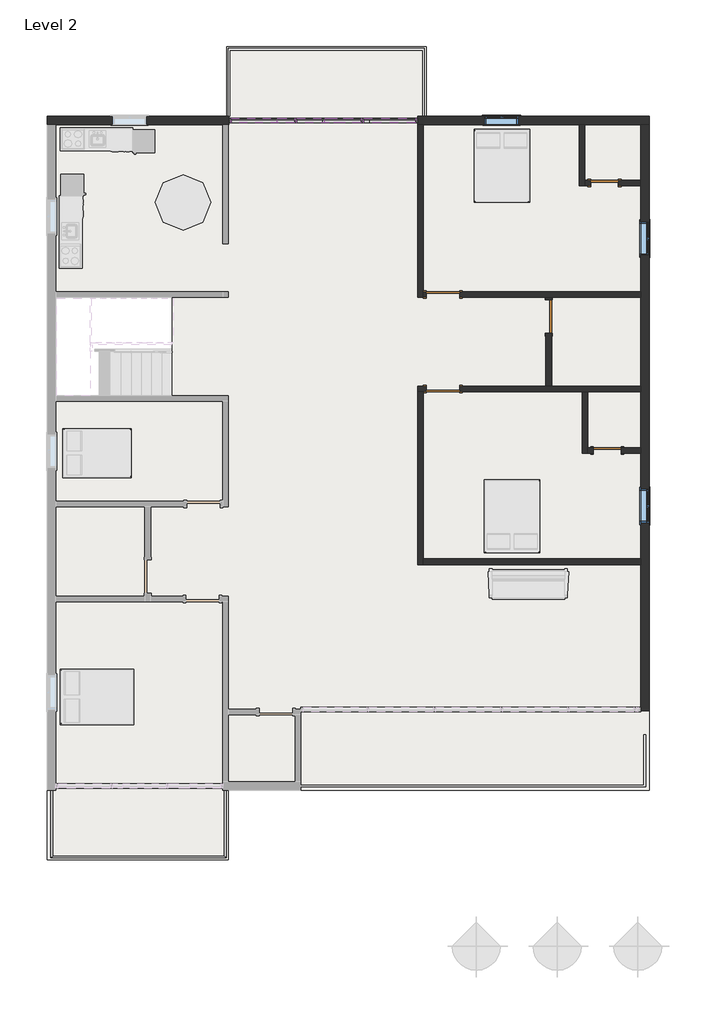
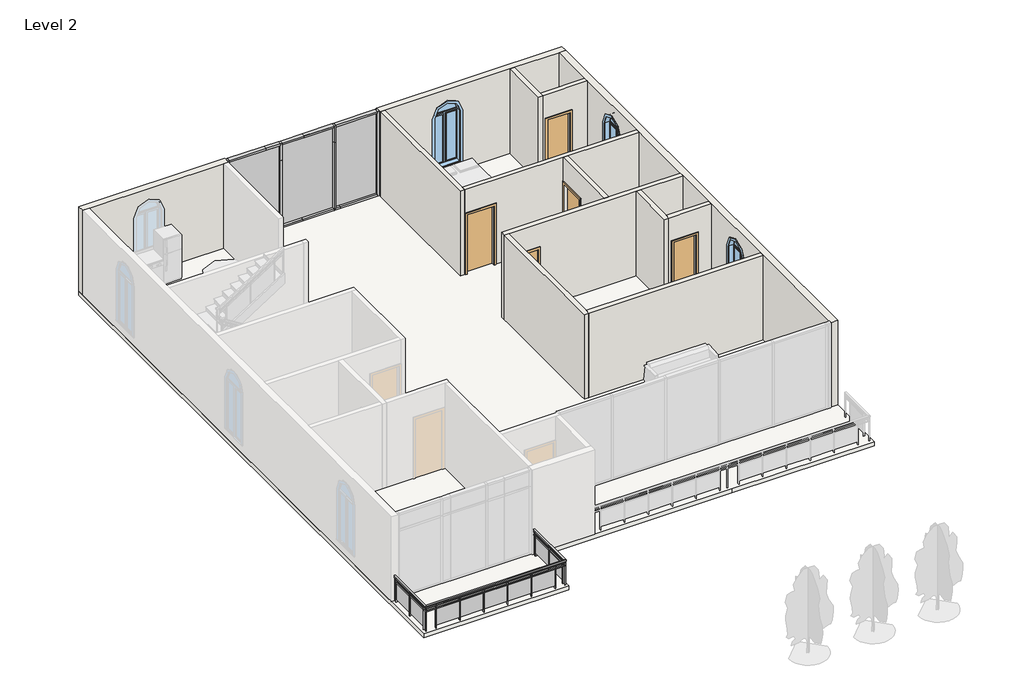
# One storey, part 2 of 3: 16 members, 13 walls, 5 doors, 3 plates, 3 windows, 1 railing, 1 slab.
"""IFC4 building model written with IfcOpenShell, lengths in millimetres."""

from ifc_helpers import new_model, si_unit, frame, origin, place, context, project, spatial, polyline, circle_curve, outline, extrude, faceted_brep, transform, mapped, element, save
from ifc_brep_helpers import plane_surface, revolved_surface, advanced_brep
from components import single_flush_2_5_e2b13fe9, door_686f89d2, door_16372e1c, member_f0fea5a5, member_f3b54ad7, member_8346ef35, member_675b1c02, member_6ed1261f, member_2238a540, member_64ee9188, member_6d5c3e5e, member_eaba9652, member_3f395ae9, system_panel_glazed_5e65faa0, system_panel_glazed_5d99744d, system_panel_glazed_395abe7e, window_e7489165

model = new_model("IFC4")

# Units and contexts
model_context = context("Model", 3, world=origin())
ifc_project = project(units=[si_unit("LENGTHUNIT", "METRE", prefix="MILLI")], contexts=[model_context])

# Site, building, storey
site = spatial("IfcSite", under=ifc_project)
building = spatial("IfcBuilding", under=site)
storey = spatial("IfcBuildingStorey", under=building, Name="Level 2", Elevation=3200.4)

# Doors
placement = place(None, origin())
single_flush_2_5_shape = single_flush_2_5_e2b13fe9(model_context)
element("IfcDoor", 1, ObjectType="Single-Flush : 2.5'", at=placement, inside=storey, context=model_context, shape_type="MappedRepresentation", body=[
    mapped(single_flush_2_5_shape, transform((6024.3292105, 3515.5144188, 3200.4), x_axis=(-1.0, 0.0, 0.0), y_axis=(0.0, -1.0, 0.0), z_axis=(0.0, 0.0, 1.0))),
])
element("IfcDoor", 2, ObjectType="Single-Flush : 2.5'", at=placement, inside=storey, context=model_context, shape_type="MappedRepresentation", body=[
    mapped(single_flush_2_5_shape, transform((5948.1292105, 10830.7144188, 3200.4), x_axis=(-1.0, 0.0, 0.0), y_axis=(0.0, -1.0, 0.0), z_axis=(0.0, 0.0, 1.0))),
])
door_shape = door_686f89d2(model_context)
element("IfcDoor", 3, ObjectType="Single-Flush : 36\" x 84\"", at=placement, inside=storey, context=model_context, shape_type="MappedRepresentation", body=[
    mapped(door_shape, transform((1528.5292105, 7782.7144188, 3200.4), x_axis=(-1.0, 0.0, 0.0), y_axis=(0.0, -1.0, 0.0), z_axis=(0.0, 0.0, 1.0))),
])
element("IfcDoor", 4, ObjectType="Single-Flush : 36\" x 84\"", at=placement, inside=storey, context=model_context, shape_type="MappedRepresentation", body=[
    mapped(door_shape, transform((4424.1292105, 7173.1144188, 3200.4), x_axis=(0.0, 1.0, 0.0), y_axis=(-1.0, 0.0, 0.0), z_axis=(0.0, 0.0, 1.0))),
])
door_2_shape = door_16372e1c(model_context)
element("IfcDoor", 5, ObjectType="Single-Flush : 36\" x 84\"", at=placement, inside=storey, context=model_context, shape_type="MappedRepresentation", body=[
    mapped(door_2_shape, transform((1528.5292105, 5191.9144188, 3200.4), x_axis=(-1.0, 0.0, 0.0), y_axis=(0.0, -1.0, 0.0), z_axis=(0.0, 0.0, 1.0))),
])

# Members
member_shape = member_f0fea5a5(model_context)
element("IfcMember", 6, ObjectType="Rectangular Mullion : 2.5\" x 5\" rectangular", at=placement, inside=storey, context=model_context, shape_type="MappedRepresentation", body=[
    mapped(member_shape, transform((-2497.3707895, 12545.2144188, 3200.4), x_axis=(1.0, 0.0, 0.0), y_axis=(0.0, -1.0, 0.0), z_axis=(0.0, 0.0, -1.0))),
])
element("IfcMember", 7, ObjectType="Rectangular Mullion : 2.5\" x 5\" rectangular", at=placement, inside=storey, context=model_context, shape_type="MappedRepresentation", body=[
    mapped(member_shape, transform((-668.5707895, 12545.2144188, 3200.4), x_axis=(1.0, 0.0, 0.0), y_axis=(0.0, -1.0, 0.0), z_axis=(0.0, 0.0, -1.0))),
])
member_2_shape = member_f3b54ad7(model_context)
element("IfcMember", 8, ObjectType="Rectangular Mullion : 2.5\" x 5\" rectangular", at=placement, inside=storey, context=model_context, shape_type="MappedRepresentation", body=[
    mapped(member_2_shape, transform((-2529.1207895, 12545.2144188, 6248.4), x_axis=(0.0, 0.0, 1.0), y_axis=(0.0, -1.0, 0.0), z_axis=(1.0, 0.0, 0.0))),
])
member_3_shape = member_8346ef35(model_context)
element("IfcMember", 9, ObjectType="Rectangular Mullion : 2.5\" x 5\" rectangular", at=placement, inside=storey, context=model_context, shape_type="MappedRepresentation", body=[
    mapped(member_3_shape, transform((-700.3207895, 12545.2144188, 6248.4), x_axis=(0.0, 0.0, 1.0), y_axis=(0.0, -1.0, 0.0), z_axis=(1.0, 0.0, 0.0))),
])
member_4_shape = member_675b1c02(model_context)
element("IfcMember", 10, ObjectType="Rectangular Mullion : 2.5\" x 5\" rectangular", at=placement, inside=storey, context=model_context, shape_type="MappedRepresentation", body=[
    mapped(member_4_shape, transform((-2465.6207895, 12545.2144188, 3200.4), x_axis=(0.0, 0.0, -1.0), y_axis=(0.0, -1.0, 0.0), z_axis=(-1.0, 0.0, 0.0))),
])
member_5_shape = member_6ed1261f(model_context)
element("IfcMember", 11, ObjectType="Rectangular Mullion : 2.5\" x 5\" rectangular", at=placement, inside=storey, context=model_context, shape_type="MappedRepresentation", body=[
    mapped(member_5_shape, transform((-636.8207895, 12545.2144188, 3200.4), x_axis=(0.0, 0.0, -1.0), y_axis=(0.0, -1.0, 0.0), z_axis=(-1.0, 0.0, 0.0))),
])
member_6_shape = member_2238a540(model_context)
element("IfcMember", 12, ObjectType="Rectangular Mullion : 2.5\" x 5\" rectangular", at=placement, inside=storey, context=model_context, shape_type="MappedRepresentation", body=[
    mapped(member_6_shape, transform((778.6208729, 12545.2144188, 6248.4), x_axis=(0.0, 0.0, 1.0), y_axis=(0.0, -1.0, 0.0), z_axis=(1.0, 0.0, 0.0))),
])
member_7_shape = member_64ee9188(model_context)
element("IfcMember", 13, ObjectType="Rectangular Mullion : 2.5\" x 5\" rectangular", at=placement, inside=storey, context=model_context, shape_type="MappedRepresentation", body=[
    mapped(member_7_shape, transform((-4262.6707895, 12545.2144188, 3200.4), x_axis=(0.0, 0.0, -1.0), y_axis=(0.0, -1.0, 0.0), z_axis=(-1.0, 0.0, 0.0))),
])
element("IfcMember", 14, ObjectType="Rectangular Mullion : 2.5\" x 5\" rectangular", at=placement, inside=storey, context=model_context, shape_type="MappedRepresentation", body=[
    mapped(member_7_shape, transform((-2529.1207895, 12545.2144188, 6248.4), x_axis=(0.0, 0.0, 1.0), y_axis=(0.0, -1.0, 0.0), z_axis=(1.0, 0.0, 0.0))),
])
member_8_shape = member_6d5c3e5e(model_context)
element("IfcMember", 15, ObjectType="Rectangular Mullion : 2.5\" x 5\" rectangular", at=placement, inside=storey, context=model_context, shape_type="MappedRepresentation", body=[
    mapped(member_8_shape, transform((-700.3207895, 12545.2144188, 6248.4), x_axis=(0.0, 0.0, 1.0), y_axis=(0.0, -1.0, 0.0), z_axis=(1.0, 0.0, 0.0))),
])
element("IfcMember", 16, ObjectType="Rectangular Mullion : 2.5\" x 5\" rectangular", at=placement, inside=storey, context=model_context, shape_type="MappedRepresentation", body=[
    mapped(member_8_shape, transform((-2465.6207895, 12545.2144188, 3200.4), x_axis=(0.0, 0.0, -1.0), y_axis=(0.0, -1.0, 0.0), z_axis=(-1.0, 0.0, 0.0))),
])
element("IfcMember", 17, ObjectType="Rectangular Mullion : 2.5\" x 5\" rectangular", at=placement, inside=storey, context=model_context, shape_type="MappedRepresentation", body=[
    mapped(member_6_shape, transform((-636.8207895, 12545.2144188, 3200.4), x_axis=(0.0, 0.0, -1.0), y_axis=(0.0, -1.0, 0.0), z_axis=(-1.0, 0.0, 0.0))),
])
member_9_shape = member_eaba9652(model_context)
element("IfcMember", 18, ObjectType="Rectangular Mullion : 2.5\" x 5\" rectangular", at=placement, inside=storey, context=model_context, shape_type="MappedRepresentation", body=[
    mapped(member_9_shape, transform((-2497.3707895, 12545.2144188, 3200.4), x_axis=(1.0, 0.0, 0.0), y_axis=(0.0, -1.0, 0.0), z_axis=(0.0, 0.0, -1.0))),
])
element("IfcMember", 19, ObjectType="Rectangular Mullion : 2.5\" x 5\" rectangular", at=placement, inside=storey, context=model_context, shape_type="MappedRepresentation", body=[
    mapped(member_9_shape, transform((-668.5707895, 12545.2144188, 3200.4), x_axis=(1.0, 0.0, 0.0), y_axis=(0.0, -1.0, 0.0), z_axis=(0.0, 0.0, -1.0))),
])
member_10_shape = member_3f395ae9(model_context)
element("IfcMember", 20, ObjectType="Rectangular Mullion : 2.5\" x 5\" rectangular", at=placement, inside=storey, context=model_context, shape_type="MappedRepresentation", body=[
    mapped(member_10_shape, transform((842.1208729, 12545.2144188, 3200.4), x_axis=(1.0, 0.0, 0.0), y_axis=(0.0, -1.0, 0.0), z_axis=(0.0, 0.0, -1.0))),
])
element("IfcMember", 21, ObjectType="Rectangular Mullion : 2.5\" x 5\" rectangular", at=placement, inside=storey, context=model_context, shape_type="MappedRepresentation", body=[
    mapped(member_10_shape, transform((-4326.1707895, 12545.2144188, 6248.4), x_axis=(-1.0, 0.0, 0.0), y_axis=(0.0, -1.0, 0.0), z_axis=(0.0, 0.0, 1.0))),
])

# Plates
system_panel_glazed_shape = system_panel_glazed_5e65faa0(model_context)
element("IfcPlate", 22, ObjectType="System Panel : Glazed", at=placement, inside=storey, context=model_context, shape_type="MappedRepresentation", body=[
    mapped(system_panel_glazed_shape, transform((-3395.8957895, 12545.2144188, 3263.9), x_axis=(1.0, 0.0, 0.0), y_axis=(0.0, 1.0, 0.0), z_axis=(0.0, 0.0, 1.0))),
])
system_panel_glazed_2_shape = system_panel_glazed_5d99744d(model_context)
element("IfcPlate", 23, ObjectType="System Panel : Glazed", at=placement, inside=storey, context=model_context, shape_type="MappedRepresentation", body=[
    mapped(system_panel_glazed_2_shape, transform((-1582.9707895, 12545.2144188, 3263.9), x_axis=(1.0, 0.0, 0.0), y_axis=(0.0, 1.0, 0.0), z_axis=(0.0, 0.0, 1.0))),
])
system_panel_glazed_3_shape = system_panel_glazed_395abe7e(model_context)
element("IfcPlate", 24, ObjectType="System Panel : Glazed", at=placement, inside=storey, context=model_context, shape_type="MappedRepresentation", body=[
    mapped(system_panel_glazed_3_shape, transform((70.9000417, 12545.2144188, 3263.9), x_axis=(1.0, 0.0, 0.0), y_axis=(0.0, 1.0, 0.0), z_axis=(0.0, 0.0, 1.0))),
])

# Railing
element("IfcRailing", 25, ObjectType="Glass Panel - Bottom Fill", at=placement, inside=storey, context=model_context, shape_type="SolidModel", body=[
    faceted_brep([(-9152.1707895, -5780.8855812, 4114.8), (-9152.1707895, -5780.8855812, 4064.0), (-9202.9707895, -5780.8855812, 4064.0), (-9202.9707895, -5780.8855812, 4114.8), (-9152.1707895, -7584.2855812, 4114.8), (-9152.1707895, -7584.2855812, 4064.0), (-9202.9707895, -7635.0855812, 4064.0), (-9202.9707895, -7635.0855812, 4114.8), (-4453.1707895, -7584.2855812, 4114.8), (-4453.1707895, -7584.2855812, 4064.0), (-4402.3707895, -7635.0855812, 4064.0), (-4402.3707895, -7635.0855812, 4114.8), (-4453.1707895, -5780.8855812, 4114.8), (-4402.3707895, -5780.8855812, 4114.8), (-4402.3707895, -5780.8855812, 4064.0), (-4453.1707895, -5780.8855812, 4064.0)], [[[0, 1, 2, 3]], [[1, 0, 4, 5]], [[2, 1, 5, 6]], [[3, 2, 6, 7]], [[0, 3, 7, 4]], [[5, 4, 8, 9]], [[6, 5, 9, 10]], [[7, 6, 10, 11]], [[4, 7, 11, 8]], [[12, 13, 14, 15]], [[9, 8, 12, 15]], [[10, 9, 15, 14]], [[11, 10, 14, 13]], [[8, 11, 13, 12]]]),
    faceted_brep([(-9190.2707895, -5780.8855812, 4025.9), (-9164.8707895, -5780.8855812, 4025.9), (-9164.8707895, -5780.8855812, 4000.5), (-9190.2707895, -5780.8855812, 4000.5), (-9190.2707895, -7622.3855812, 4025.9), (-9164.8707895, -7596.9855812, 4025.9), (-9164.8707895, -7596.9855812, 4000.5), (-9190.2707895, -7622.3855812, 4000.5), (-4415.0707895, -7622.3855812, 4025.9), (-4440.4707895, -7596.9855812, 4025.9), (-4440.4707895, -7596.9855812, 4000.5), (-4415.0707895, -7622.3855812, 4000.5), (-4415.0707895, -5780.8855812, 4025.9), (-4415.0707895, -5780.8855812, 4000.5), (-4440.4707895, -5780.8855812, 4000.5), (-4440.4707895, -5780.8855812, 4025.9)], [[[0, 1, 2, 3]], [[1, 0, 4, 5]], [[2, 1, 5, 6]], [[3, 2, 6, 7]], [[0, 3, 7, 4]], [[5, 4, 8, 9]], [[6, 5, 9, 10]], [[7, 6, 10, 11]], [[4, 7, 11, 8]], [[12, 13, 14, 15]], [[9, 8, 12, 15]], [[10, 9, 15, 14]], [[11, 10, 14, 13]], [[8, 11, 13, 12]]]),
    faceted_brep([(-9190.2707895, -5780.8855812, 3924.3), (-9164.8707895, -5780.8855812, 3924.3), (-9164.8707895, -5780.8855812, 3898.9), (-9190.2707895, -5780.8855812, 3898.9), (-9190.2707895, -7622.3855812, 3924.3), (-9164.8707895, -7596.9855812, 3924.3), (-9164.8707895, -7596.9855812, 3898.9), (-9190.2707895, -7622.3855812, 3898.9), (-4415.0707895, -7622.3855812, 3924.3), (-4440.4707895, -7596.9855812, 3924.3), (-4440.4707895, -7596.9855812, 3898.9), (-4415.0707895, -7622.3855812, 3898.9), (-4415.0707895, -5780.8855812, 3924.3), (-4415.0707895, -5780.8855812, 3898.9), (-4440.4707895, -5780.8855812, 3898.9), (-4440.4707895, -5780.8855812, 3924.3)], [[[0, 1, 2, 3]], [[1, 0, 4, 5]], [[2, 1, 5, 6]], [[3, 2, 6, 7]], [[0, 3, 7, 4]], [[5, 4, 8, 9]], [[6, 5, 9, 10]], [[7, 6, 10, 11]], [[4, 7, 11, 8]], [[12, 13, 14, 15]], [[9, 8, 12, 15]], [[10, 9, 15, 14]], [[11, 10, 14, 13]], [[8, 11, 13, 12]]]),
    extrude(outline(polyline([(-4402.3707895, -5888.8355812), (-4453.1707895, -5888.8355812), (-4453.1707895, -5876.1355812), (-4402.3707895, -5876.1355812), (-4402.3707895, -5888.8355812)])), frame((0.0, 0.0, 3200.4), z_axis=(0.0, 0.0, 1.0), x_axis=(1.0, 0.0, 0.0)), (0.0, 0.0, 1.0), 863.6),
    extrude(outline(polyline([(-4434.3059465, -6695.2855812), (-4434.3059465, -5882.4855812), (-4427.9559465, -5882.4855812), (-4427.9559465, -6695.2855812), (-4434.3059465, -6695.2855812)])), frame((0.0, 0.0, 3302.0), z_axis=(0.0, 0.0, 1.0), x_axis=(1.0, 0.0, 0.0)), (0.0, 0.0, 1.0), 596.9),
    extrude(outline(polyline([(-4402.3707895, -6701.6355812), (-4453.1707895, -6701.6355812), (-4453.1707895, -6688.9355812), (-4402.3707895, -6688.9355812), (-4402.3707895, -6701.6355812)])), frame((0.0, 0.0, 3200.4), z_axis=(0.0, 0.0, 1.0), x_axis=(1.0, 0.0, 0.0)), (0.0, 0.0, 1.0), 863.6),
    extrude(outline(polyline([(-4434.3059465, -7508.0855812), (-4434.3059465, -6695.2855812), (-4427.9559465, -6695.2855812), (-4427.9559465, -7508.0855812), (-4434.3059465, -7508.0855812)])), frame((0.0, 0.0, 3302.0), z_axis=(0.0, 0.0, 1.0), x_axis=(1.0, 0.0, 0.0)), (0.0, 0.0, 1.0), 596.9),
    extrude(outline(polyline([(-4402.3707895, -7514.4355812), (-4453.1707895, -7514.4355812), (-4453.1707895, -7501.7355812), (-4402.3707895, -7501.7355812), (-4402.3707895, -7514.4355812)])), frame((0.0, 0.0, 3200.4), z_axis=(0.0, 0.0, 1.0), x_axis=(1.0, 0.0, 0.0)), (0.0, 0.0, 1.0), 863.6),
    extrude(outline(polyline([(-4777.0207895, -7635.0855812), (-4777.0207895, -7584.2855812), (-4764.3207895, -7584.2855812), (-4764.3207895, -7635.0855812), (-4777.0207895, -7635.0855812)])), frame((0.0, 0.0, 3200.4), z_axis=(0.0, 0.0, 1.0), x_axis=(1.0, 0.0, 0.0)), (0.0, 0.0, 1.0), 863.6),
    extrude(outline(polyline([(-5583.4707895, -7603.1504242), (-4770.6707895, -7603.1504242), (-4770.6707895, -7609.5004242), (-5583.4707895, -7609.5004242), (-5583.4707895, -7603.1504242)])), frame((0.0, 0.0, 3302.0), z_axis=(0.0, 0.0, 1.0), x_axis=(1.0, 0.0, 0.0)), (0.0, 0.0, 1.0), 596.9),
    extrude(outline(polyline([(-5589.8207895, -7635.0855812), (-5589.8207895, -7584.2855812), (-5577.1207895, -7584.2855812), (-5577.1207895, -7635.0855812), (-5589.8207895, -7635.0855812)])), frame((0.0, 0.0, 3200.4), z_axis=(0.0, 0.0, 1.0), x_axis=(1.0, 0.0, 0.0)), (0.0, 0.0, 1.0), 863.6),
    extrude(outline(polyline([(-6396.2707895, -7603.1504242), (-5583.4707895, -7603.1504242), (-5583.4707895, -7609.5004242), (-6396.2707895, -7609.5004242), (-6396.2707895, -7603.1504242)])), frame((0.0, 0.0, 3302.0), z_axis=(0.0, 0.0, 1.0), x_axis=(1.0, 0.0, 0.0)), (0.0, 0.0, 1.0), 596.9),
    extrude(outline(polyline([(-6402.6207895, -7635.0855812), (-6402.6207895, -7584.2855812), (-6389.9207895, -7584.2855812), (-6389.9207895, -7635.0855812), (-6402.6207895, -7635.0855812)])), frame((0.0, 0.0, 3200.4), z_axis=(0.0, 0.0, 1.0), x_axis=(1.0, 0.0, 0.0)), (0.0, 0.0, 1.0), 863.6),
    extrude(outline(polyline([(-7209.0707895, -7603.1504242), (-6396.2707895, -7603.1504242), (-6396.2707895, -7609.5004242), (-7209.0707895, -7609.5004242), (-7209.0707895, -7603.1504242)])), frame((0.0, 0.0, 3302.0), z_axis=(0.0, 0.0, 1.0), x_axis=(1.0, 0.0, 0.0)), (0.0, 0.0, 1.0), 596.9),
    extrude(outline(polyline([(-7215.4207895, -7635.0855812), (-7215.4207895, -7584.2855812), (-7202.7207895, -7584.2855812), (-7202.7207895, -7635.0855812), (-7215.4207895, -7635.0855812)])), frame((0.0, 0.0, 3200.4), z_axis=(0.0, 0.0, 1.0), x_axis=(1.0, 0.0, 0.0)), (0.0, 0.0, 1.0), 863.6),
    extrude(outline(polyline([(-8021.8707895, -7603.1504242), (-7209.0707895, -7603.1504242), (-7209.0707895, -7609.5004242), (-8021.8707895, -7609.5004242), (-8021.8707895, -7603.1504242)])), frame((0.0, 0.0, 3302.0), z_axis=(0.0, 0.0, 1.0), x_axis=(1.0, 0.0, 0.0)), (0.0, 0.0, 1.0), 596.9),
    extrude(outline(polyline([(-8028.2207895, -7635.0855812), (-8028.2207895, -7584.2855812), (-8015.5207895, -7584.2855812), (-8015.5207895, -7635.0855812), (-8028.2207895, -7635.0855812)])), frame((0.0, 0.0, 3200.4), z_axis=(0.0, 0.0, 1.0), x_axis=(1.0, 0.0, 0.0)), (0.0, 0.0, 1.0), 863.6),
    extrude(outline(polyline([(-8834.6707895, -7603.1504242), (-8021.8707895, -7603.1504242), (-8021.8707895, -7609.5004242), (-8834.6707895, -7609.5004242), (-8834.6707895, -7603.1504242)])), frame((0.0, 0.0, 3302.0), z_axis=(0.0, 0.0, 1.0), x_axis=(1.0, 0.0, 0.0)), (0.0, 0.0, 1.0), 596.9),
    extrude(outline(polyline([(-8841.0207895, -7635.0855812), (-8841.0207895, -7584.2855812), (-8828.3207895, -7584.2855812), (-8828.3207895, -7635.0855812), (-8841.0207895, -7635.0855812)])), frame((0.0, 0.0, 3200.4), z_axis=(0.0, 0.0, 1.0), x_axis=(1.0, 0.0, 0.0)), (0.0, 0.0, 1.0), 863.6),
    extrude(outline(polyline([(-9202.9707895, -7501.7355812), (-9152.1707895, -7501.7355812), (-9152.1707895, -7514.4355812), (-9202.9707895, -7514.4355812), (-9202.9707895, -7501.7355812)])), frame((0.0, 0.0, 3200.4), z_axis=(0.0, 0.0, 1.0), x_axis=(1.0, 0.0, 0.0)), (0.0, 0.0, 1.0), 863.6),
    extrude(outline(polyline([(-9171.0356325, -6695.2855812), (-9171.0356325, -7508.0855812), (-9177.3856325, -7508.0855812), (-9177.3856325, -6695.2855812), (-9171.0356325, -6695.2855812)])), frame((0.0, 0.0, 3302.0), z_axis=(0.0, 0.0, 1.0), x_axis=(1.0, 0.0, 0.0)), (0.0, 0.0, 1.0), 596.9),
    extrude(outline(polyline([(-9202.9707895, -6688.9355812), (-9152.1707895, -6688.9355812), (-9152.1707895, -6701.6355812), (-9202.9707895, -6701.6355812), (-9202.9707895, -6688.9355812)])), frame((0.0, 0.0, 3200.4), z_axis=(0.0, 0.0, 1.0), x_axis=(1.0, 0.0, 0.0)), (0.0, 0.0, 1.0), 863.6),
    extrude(outline(polyline([(-9171.0356325, -5882.4855812), (-9171.0356325, -6695.2855812), (-9177.3856325, -6695.2855812), (-9177.3856325, -5882.4855812), (-9171.0356325, -5882.4855812)])), frame((0.0, 0.0, 3302.0), z_axis=(0.0, 0.0, 1.0), x_axis=(1.0, 0.0, 0.0)), (0.0, 0.0, 1.0), 596.9),
    extrude(outline(polyline([(-9202.9707895, -5876.1355812), (-9152.1707895, -5876.1355812), (-9152.1707895, -5888.8355812), (-9202.9707895, -5888.8355812), (-9202.9707895, -5876.1355812)])), frame((0.0, 0.0, 3200.4), z_axis=(0.0, 0.0, 1.0), x_axis=(1.0, 0.0, 0.0)), (0.0, 0.0, 1.0), 863.6),
    extrude(outline(polyline([(-4437.2957895, -7619.2105812), (-4437.2957895, -7600.1605812), (-4418.2457895, -7600.1605812), (-4418.2457895, -7619.2105812), (-4437.2957895, -7619.2105812)])), frame((0.0, 0.0, 3200.4), z_axis=(0.0, 0.0, 1.0), x_axis=(1.0, 0.0, 0.0)), (0.0, 0.0, 1.0), 863.6),
    extrude(outline(polyline([(-9187.0957895, -7600.1605812), (-9168.0457895, -7600.1605812), (-9168.0457895, -7619.2105812), (-9187.0957895, -7619.2105812), (-9187.0957895, -7600.1605812)])), frame((0.0, 0.0, 3200.4), z_axis=(0.0, 0.0, 1.0), x_axis=(1.0, 0.0, 0.0)), (0.0, 0.0, 1.0), 863.6),
    extrude(outline(polyline([(-4418.2457895, -5793.5855812), (-4437.2957895, -5793.5855812), (-4437.2957895, -5774.5355812), (-4418.2457895, -5774.5355812), (-4418.2457895, -5793.5855812)])), frame((0.0, 0.0, 3200.4), z_axis=(0.0, 0.0, 1.0), x_axis=(1.0, 0.0, 0.0)), (0.0, 0.0, 1.0), 863.6),
    extrude(outline(polyline([(-9187.0957895, -5774.5355812), (-9168.0457895, -5774.5355812), (-9168.0457895, -5793.5855812), (-9187.0957895, -5793.5855812), (-9187.0957895, -5774.5355812)])), frame((0.0, 0.0, 3200.4), z_axis=(0.0, 0.0, 1.0), x_axis=(1.0, 0.0, 0.0)), (0.0, 0.0, 1.0), 863.6),
])

# Slab
element("IfcSlab", 26, ObjectType="6\"", at=placement, inside=storey, context=model_context, shape_type="SweptSolid", body=[
    extrude(outline(polyline([(-9292.4791271, -7685.8046952), (-9292.4791271, 12659.5144188), (-4390.2791271, 12659.5144188), (-4390.2791271, 14564.5144188), (1070.7208729, 14564.5144188), (1070.7208729, 12659.5953048), (7167.3292105, 12659.5953048), (7167.3292105, -4256.8046952), (7167.3292105, -5780.8046952), (2315.3208729, -5780.8046952), (-4339.4791271, -5780.8046952), (-4339.4791271, -7685.8046952), (-9292.4791271, -7685.8046952)]), holes=[polyline([(-5888.2707895, 7706.5953048), (-9063.8791271, 7706.5953048), (-9063.8791271, 5014.1144188), (-5888.2707895, 5014.1144188), (-5888.2707895, 7706.5953048)])]), frame((0.0, 0.0, 3048.0), z_axis=(0.0, 0.0, 1.0), x_axis=(1.0, 0.0, 0.0)), (0.0, 0.0, 1.0), 152.4),
])

# Walls
element("IfcWall", 27, ObjectType="6\"", at=placement, inside=storey, context=model_context, shape_type="Brep", body=[
    faceted_brep([(842.7292105, 12430.9144188, 3200.4), (842.7292105, 7706.5144188, 3200.4), (842.7292105, 7706.5144188, 6248.4), (842.7292105, 12430.9144188, 6248.4), (995.1292105, 12430.9144188, 3200.4), (995.1292105, 12430.9144188, 6248.4), (995.1292105, 7858.9144188, 6248.4), (995.1292105, 7706.5144188, 6248.4), (995.1292105, 7706.5144188, 3200.4), (995.1292105, 7858.9144188, 3200.4)], [[[0, 1, 2, 3]], [[4, 5, 6, 7, 8, 9]], [[1, 0, 4, 9, 8]], [[3, 2, 7, 6, 5]], [[0, 3, 5, 4]], [[2, 1, 8, 7]]]),
])
element("IfcWall", 28, ObjectType="6\"", at=placement, inside=storey, context=model_context, shape_type="Brep", body=[
    faceted_brep([(995.1292105, 7706.5144188, 3200.4), (1071.3292105, 7706.5144188, 3200.4), (1071.3292105, 7706.5144188, 5334.0), (1985.7292105, 7706.5144188, 5334.0), (1985.7292105, 7706.5144188, 3200.4), (4347.9292105, 7706.5144188, 3200.4), (4500.3292105, 7706.5144188, 3200.4), (6938.7292105, 7706.5144188, 3200.4), (6938.7292105, 7706.5144188, 6248.4), (4500.3292105, 7706.5144188, 6248.4), (4347.9292105, 7706.5144188, 6248.4), (995.1292105, 7706.5144188, 6248.4), (1071.3292105, 7858.9144188, 5334.0), (1071.3292105, 7858.9144188, 3200.4), (995.1292105, 7858.9144188, 3200.4), (995.1292105, 7858.9144188, 6248.4), (6938.7292105, 7858.9144188, 6248.4), (6938.7292105, 7858.9144188, 3200.4), (1985.7292105, 7858.9144188, 3200.4), (1985.7292105, 7858.9144188, 5334.0)], [[[0, 1, 2, 3, 4, 5, 6, 7, 8, 9, 10, 11]], [[12, 13, 14, 15, 16, 17, 18, 19]], [[18, 17, 7, 6, 5, 4]], [[14, 13, 1, 0]], [[11, 10, 9, 8, 16, 15]], [[0, 11, 15, 14]], [[8, 7, 17, 16]], [[2, 1, 13, 12]], [[3, 2, 12, 19]], [[4, 3, 19, 18]]]),
])
element("IfcWall", 29, ObjectType="6\"", at=placement, inside=storey, context=model_context, shape_type="Brep", body=[
    faceted_brep([(1071.3292105, 5268.1144188, 5334.0), (1071.3292105, 5268.1144188, 3200.4), (842.7292105, 5268.1144188, 3200.4), (842.7292105, 5268.1144188, 6248.4), (4347.9292105, 5268.1144188, 6248.4), (4500.3292105, 5268.1144188, 6248.4), (6938.7292105, 5268.1144188, 6248.4), (6938.7292105, 5268.1144188, 3200.4), (4500.3292105, 5268.1144188, 3200.4), (4347.9292105, 5268.1144188, 3200.4), (1985.7292105, 5268.1144188, 3200.4), (1985.7292105, 5268.1144188, 5334.0), (842.7292105, 5115.7144188, 3200.4), (995.1292105, 5115.7144188, 3200.4), (1071.3292105, 5115.7144188, 3200.4), (1071.3292105, 5115.7144188, 5334.0), (1985.7292105, 5115.7144188, 5334.0), (1985.7292105, 5115.7144188, 3200.4), (5338.5292105, 5115.7144188, 3200.4), (5490.9292105, 5115.7144188, 3200.4), (6938.7292105, 5115.7144188, 3200.4), (6938.7292105, 5115.7144188, 6248.4), (5490.9292105, 5115.7144188, 6248.4), (5338.5292105, 5115.7144188, 6248.4), (995.1292105, 5115.7144188, 6248.4), (842.7292105, 5115.7144188, 6248.4)], [[[0, 1, 2, 3, 4, 5, 6, 7, 8, 9, 10, 11]], [[12, 13, 14, 15, 16, 17, 18, 19, 20, 21, 22, 23, 24, 25]], [[2, 1, 14, 13, 12]], [[10, 9, 8, 7, 20, 19, 18, 17]], [[6, 5, 4, 3, 25, 24, 23, 22, 21]], [[7, 6, 21, 20]], [[3, 2, 12, 25]], [[15, 14, 1, 0]], [[16, 15, 0, 11]], [[17, 16, 11, 10]]]),
])
element("IfcWall", 30, ObjectType="6\"", at=placement, inside=storey, context=model_context, shape_type="SweptSolid", body=[
    extrude(outline(polyline([(7706.5144188, 3200.4), (7630.3144188, 3200.4), (7630.3144188, 5334.0), (6715.9144188, 5334.0), (6715.9144188, 3200.4), (5268.1144188, 3200.4), (5268.1144188, 6248.4), (7706.5144188, 6248.4), (7706.5144188, 3200.4)])), frame((4347.9292105, 0.0, 0.0), z_axis=(1.0, 0.0, 0.0), x_axis=(0.0, 1.0, 0.0)), (0.0, 0.0, 1.0), 152.4),
])
element("IfcWall", 31, ObjectType="6\"", at=placement, inside=storey, context=model_context, shape_type="Brep", body=[
    faceted_brep([(842.7292105, 5115.7144188, 3200.4), (842.7292105, 391.3144188, 3200.4), (842.7292105, 391.3144188, 6248.4), (842.7292105, 5115.7144188, 6248.4), (995.1292105, 5115.7144188, 3200.4), (995.1292105, 5115.7144188, 6248.4), (995.1292105, 543.7144188, 6248.4), (995.1292105, 391.3144188, 6248.4), (995.1292105, 391.3144188, 3200.4), (995.1292105, 543.7144188, 3200.4)], [[[0, 1, 2, 3]], [[4, 5, 6, 7, 8, 9]], [[1, 0, 4, 9, 8]], [[3, 2, 7, 6, 5]], [[2, 1, 8, 7]], [[0, 3, 5, 4]]]),
])
element("IfcWall", 32, ObjectType="6\"", at=placement, inside=storey, context=model_context, shape_type="SweptSolid", body=[
    extrude(outline(polyline([(6938.7292105, 391.3144188), (995.1292105, 391.3144188), (995.1292105, 543.7144188), (6938.7292105, 543.7144188), (6938.7292105, 391.3144188)])), frame((0.0, 0.0, 3200.4), z_axis=(0.0, 0.0, 1.0), x_axis=(1.0, 0.0, 0.0)), (0.0, 0.0, 1.0), 3048.0),
])
element("IfcWall", 33, ObjectType="6\"", at=placement, inside=storey, context=model_context, shape_type="Brep", body=[
    faceted_brep([(5262.3292105, 12430.9144188, 3200.4), (5262.3292105, 10754.5144188, 3200.4), (5262.3292105, 10754.5144188, 6248.4), (5262.3292105, 12430.9144188, 6248.4), (5414.7292105, 12430.9144188, 3200.4), (5414.7292105, 12430.9144188, 6248.4), (5414.7292105, 10906.9144188, 6248.4), (5414.7292105, 10754.5144188, 6248.4), (5414.7292105, 10754.5144188, 3200.4), (5414.7292105, 10906.9144188, 3200.4)], [[[0, 1, 2, 3]], [[4, 5, 6, 7, 8, 9]], [[1, 0, 4, 9, 8]], [[3, 2, 7, 6, 5]], [[0, 3, 5, 4]], [[2, 1, 8, 7]]]),
])
element("IfcWall", 34, ObjectType="6\"", at=placement, inside=storey, context=model_context, shape_type="SweptSolid", body=[
    extrude(outline(polyline([(3200.4, 5414.7292105), (3200.4, 5567.1292105), (5334.0, 5567.1292105), (5334.0, 6329.1292105), (3200.4, 6329.1292105), (3200.4, 6938.7292105), (6248.4, 6938.7292105), (6248.4, 5414.7292105), (3200.4, 5414.7292105)])), frame((0.0, 10754.5144188, 0.0), z_axis=(0.0, 1.0, 0.0), x_axis=(0.0, 0.0, 1.0)), (0.0, 0.0, 1.0), 152.4),
])
element("IfcWall", 35, ObjectType="6\"", at=placement, inside=storey, context=model_context, shape_type="Brep", body=[
    faceted_brep([(5338.5292105, 5115.7144188, 3200.4), (5338.5292105, 3439.3144188, 3200.4), (5338.5292105, 3439.3144188, 6248.4), (5338.5292105, 5115.7144188, 6248.4), (5490.9292105, 5115.7144188, 3200.4), (5490.9292105, 5115.7144188, 6248.4), (5490.9292105, 3591.7144188, 6248.4), (5490.9292105, 3439.3144188, 6248.4), (5490.9292105, 3439.3144188, 3200.4), (5490.9292105, 3591.7144188, 3200.4)], [[[0, 1, 2, 3]], [[4, 5, 6, 7, 8, 9]], [[1, 0, 4, 9, 8]], [[3, 2, 7, 6, 5]], [[0, 3, 5, 4]], [[2, 1, 8, 7]]]),
])
element("IfcWall", 36, ObjectType="6\"", at=placement, inside=storey, context=model_context, shape_type="SweptSolid", body=[
    extrude(outline(polyline([(3200.4, 5490.9292105), (3200.4, 5643.3292105), (5334.0, 5643.3292105), (5334.0, 6405.3292105), (3200.4, 6405.3292105), (3200.4, 6938.7292105), (6248.4, 6938.7292105), (6248.4, 5490.9292105), (3200.4, 5490.9292105)])), frame((0.0, 3439.3144188, 0.0), z_axis=(0.0, 1.0, 0.0), x_axis=(0.0, 0.0, 1.0)), (0.0, 0.0, 1.0), 152.4),
])
element("IfcWall", 37, ObjectType="9\"", at=placement, inside=storey, context=model_context, shape_type="AdvancedBrep", body=[
    advanced_brep(
    [(-9291.8707895, 12430.9144188, 3200.4), (-9063.2707895, 12430.9144188, 3200.4), (-4491.2707895, 12430.9144188, 3200.4), (-4338.8707895, 12430.9144188, 3200.4), (-4326.1707895, 12430.9144188, 3200.4), (-4326.1707895, 12430.9144188, 6248.4), (-4338.8707895, 12430.9144188, 6248.4), (-4491.2707895, 12430.9144188, 6248.4), (-9063.2707895, 12430.9144188, 6248.4), (-9291.8707895, 12430.9144188, 6248.4), (-6586.7707895, 12430.9144188, 5353.05), (-6586.7707895, 12430.9144188, 3505.2), (-7501.1707895, 12430.9144188, 3505.2), (-7501.1707895, 12430.9144188, 5353.05), (-9291.8707895, 12659.5144188, 3200.4), (-9291.8707895, 12659.5144188, 6248.4), (-4326.1707895, 12659.5144188, 6248.4), (-4326.1707895, 12659.5144188, 3200.4), (-6586.7707895, 12659.5144188, 5353.05), (-7501.1707895, 12659.5144188, 5353.05), (-7501.1707895, 12659.5144188, 3505.2), (-6586.7707895, 12659.5144188, 3505.2)],
    [
        (0, 1),
        (1, 2),
        (2, 3),
        (3, 4),
        (4, 5),
        (5, 6),
        (6, 7),
        (7, 8),
        (8, 9),
        (9, 0),
        (10, 11),
        (11, 12),
        (12, 13),
        (13, 10, circle_curve(frame((-7043.9707895, 12430.9144188, 5353.05), z_axis=(0.0, 1.0, 0.0), x_axis=(1.0, 0.0, 0.0)), 457.2)),
        (14, 15),
        (15, 16),
        (16, 17),
        (17, 14),
        (18, 19, circle_curve(frame((-7043.9707895, 12659.5144188, 5353.05), z_axis=(0.0, -1.0, 0.0), x_axis=(1.0, 0.0, 0.0)), 457.2)),
        (19, 20),
        (20, 21),
        (21, 18),
        (0, 14),
        (17, 4),
        (16, 5),
        (15, 9),
        (10, 18),
        (21, 11),
        (20, 12),
        (19, 13),
    ],
    [
        plane_surface(frame((-10130.0707895, 12430.9144188, 3200.4), z_axis=(0.0, -1.0, 0.0), x_axis=(1.0, 0.0, 0.0))),
        plane_surface(frame((-10130.0707895, 12659.5144188, 3200.4), z_axis=(0.0, 1.0, 0.0), x_axis=(-1.0, 0.0, 0.0))),
        plane_surface(frame((-9177.5707895, 12430.9144188, 3200.4), z_axis=(0.0, 0.0, -1.0), x_axis=(0.0, 1.0, 0.0))),
        plane_surface(frame((-4326.1707895, 12430.9144188, 3200.4), z_axis=(1.0, 0.0, 0.0), x_axis=(0.0, 1.0, 0.0))),
        plane_surface(frame((-4326.1707895, 12430.9144188, 6248.4), z_axis=(0.0, 0.0, 1.0), x_axis=(0.0, 1.0, 0.0))),
        plane_surface(frame((-6586.7707895, 12430.9144188, 5353.05), z_axis=(-1.0, 0.0, 0.0), x_axis=(0.0, 1.0, 0.0))),
        plane_surface(frame((-6586.7707895, 12430.9144188, 3505.2), z_axis=(0.0, 0.0, 1.0), x_axis=(0.0, 1.0, 0.0))),
        plane_surface(frame((-7501.1707895, 12430.9144188, 3505.2), z_axis=(1.0, 0.0, 0.0), x_axis=(0.0, 1.0, 0.0))),
        revolved_surface(polyline([(-6586.7707895, 12659.5144188, 5353.05), (-6586.7707895, 12430.9144188, 5353.05)]), (-7043.9707895, 12430.9144188, 5353.05), (0.0, 1.0, 0.0)),
        plane_surface(frame((-9291.8707895, 12430.9144188, 3200.4), z_axis=(-1.0, 0.0, 0.0), x_axis=(0.0, -1.0, 0.0))),
    ],
    [
        (0, [[1, 2, 3, 4, 5, 6, 7, 8, 9, 10], [11, 12, 13, 14]]),
        (1, [[15, 16, 17, 18], [19, 20, 21, 22]]),
        (2, [[-4, -3, -2, -1, 23, -18, 24]]),
        (3, [[-5, -24, -17, 25]]),
        (4, [[-9, -8, -7, -6, -25, -16, 26]]),
        (5, [[-11, 27, -22, 28]]),
        (6, [[-12, -28, -21, 29]]),
        (7, [[-13, -29, -20, 30]]),
        (8, [[-14, -30, -19, -27]]),
        (9, [[-10, -26, -15, -23]]),
    ],
),
])
element("IfcWall", 38, ObjectType="9\"", at=placement, inside=storey, context=model_context, shape_type="AdvancedBrep", body=[
    advanced_brep(
    [(6938.7292105, 12430.9144188, 3200.4), (6938.7292105, 10906.9144188, 3200.4), (6938.7292105, 10754.5144188, 3200.4), (6938.7292105, 7858.9144188, 3200.4), (6938.7292105, 7706.5144188, 3200.4), (6938.7292105, 5268.1144188, 3200.4), (6938.7292105, 5115.7144188, 3200.4), (6938.7292105, 3591.7144188, 3200.4), (6938.7292105, 3439.3144188, 3200.4), (6938.7292105, 543.7144188, 3200.4), (6938.7292105, 391.3144188, 3200.4), (6938.7292105, -3606.0105812, 3200.4), (6938.7292105, -3606.0105812, 6248.4), (6938.7292105, 391.3144188, 6248.4), (6938.7292105, 543.7144188, 6248.4), (6938.7292105, 3439.3144188, 6248.4), (6938.7292105, 3591.7144188, 6248.4), (6938.7292105, 5115.7144188, 6248.4), (6938.7292105, 5268.1144188, 6248.4), (6938.7292105, 7706.5144188, 6248.4), (6938.7292105, 7858.9144188, 6248.4), (6938.7292105, 10754.5144188, 6248.4), (6938.7292105, 10906.9144188, 6248.4), (6938.7292105, 12430.9144188, 6248.4), (6938.7292105, 8852.6894188, 5353.05), (6938.7292105, 8852.6894188, 3505.2), (6938.7292105, 9767.0894188, 3505.2), (6938.7292105, 9767.0894188, 5353.05), (6938.7292105, 1537.4894188, 5353.05), (6938.7292105, 1537.4894188, 3505.2), (6938.7292105, 2451.8894188, 3505.2), (6938.7292105, 2451.8894188, 5353.05), (7167.3292105, 12430.9144188, 3200.4), (7167.3292105, 12430.9144188, 6248.4), (7167.3292105, -3606.0105812, 6248.4), (7167.3292105, -3606.0105812, 3200.4), (7167.3292105, 8852.6894188, 5353.05), (7167.3292105, 9767.0894188, 5353.05), (7167.3292105, 9767.0894188, 3505.2), (7167.3292105, 8852.6894188, 3505.2), (7167.3292105, 1537.4894188, 5353.05), (7167.3292105, 2451.8894188, 5353.05), (7167.3292105, 2451.8894188, 3505.2), (7167.3292105, 1537.4894188, 3505.2)],
    [
        (0, 1),
        (1, 2),
        (2, 3),
        (3, 4),
        (4, 5),
        (5, 6),
        (6, 7),
        (7, 8),
        (8, 9),
        (9, 10),
        (10, 11),
        (11, 12),
        (12, 13),
        (13, 14),
        (14, 15),
        (15, 16),
        (16, 17),
        (17, 18),
        (18, 19),
        (19, 20),
        (20, 21),
        (21, 22),
        (22, 23),
        (23, 0),
        (24, 25),
        (25, 26),
        (26, 27),
        (27, 24, circle_curve(frame((6938.7292105, 9309.8894188, 5353.05), z_axis=(1.0, 0.0, 0.0), x_axis=(0.0, -1.0, 0.0)), 457.2)),
        (28, 29),
        (29, 30),
        (30, 31),
        (31, 28, circle_curve(frame((6938.7292105, 1994.6894188, 5353.05), z_axis=(1.0, 0.0, 0.0), x_axis=(0.0, -1.0, 0.0)), 457.2)),
        (32, 33),
        (33, 34),
        (34, 35),
        (35, 32),
        (36, 37, circle_curve(frame((7167.3292105, 9309.8894188, 5353.05), z_axis=(-1.0, 0.0, 0.0), x_axis=(0.0, -1.0, 0.0)), 457.2)),
        (37, 38),
        (38, 39),
        (39, 36),
        (40, 41, circle_curve(frame((7167.3292105, 1994.6894188, 5353.05), z_axis=(-1.0, 0.0, 0.0), x_axis=(0.0, -1.0, 0.0)), 457.2)),
        (41, 42),
        (42, 43),
        (43, 40),
        (0, 32),
        (35, 11),
        (34, 12),
        (33, 23),
        (24, 36),
        (39, 25),
        (38, 26),
        (37, 27),
        (28, 40),
        (43, 29),
        (42, 30),
        (41, 31),
    ],
    [
        plane_surface(frame((6938.7292105, 12434.0894188, 3200.4), z_axis=(-1.0, 0.0, 0.0), x_axis=(0.0, -1.0, 0.0))),
        plane_surface(frame((7167.3292105, 12434.0894188, 3200.4), z_axis=(1.0, 0.0, 0.0), x_axis=(0.0, 1.0, 0.0))),
        plane_surface(frame((6938.7292105, 12545.2144188, 3200.4), z_axis=(0.0, 0.0, -1.0), x_axis=(1.0, 0.0, 0.0))),
        plane_surface(frame((6938.7292105, -3606.0105812, 3200.4), z_axis=(0.0, -1.0, 0.0), x_axis=(1.0, 0.0, 0.0))),
        plane_surface(frame((6938.7292105, -3606.0105812, 6248.4), z_axis=(0.0, 0.0, 1.0), x_axis=(1.0, 0.0, 0.0))),
        plane_surface(frame((6938.7292105, 8852.6894188, 5353.05), z_axis=(0.0, 1.0, 0.0), x_axis=(1.0, 0.0, 0.0))),
        plane_surface(frame((6938.7292105, 8852.6894188, 3505.2), z_axis=(0.0, 0.0, 1.0), x_axis=(1.0, 0.0, 0.0))),
        plane_surface(frame((6938.7292105, 9767.0894188, 3505.2), z_axis=(0.0, -1.0, 0.0), x_axis=(1.0, 0.0, 0.0))),
        revolved_surface(polyline([(7167.3292105, 8852.689418799999, 5353.05), (6938.7292105, 8852.689418799999, 5353.05)]), (6938.7292105, 9309.8894188, 5353.05), (1.0, 0.0, 0.0)),
        plane_surface(frame((6938.7292105, 1537.4894188, 5353.05), z_axis=(0.0, 1.0, 0.0), x_axis=(1.0, 0.0, 0.0))),
        plane_surface(frame((6938.7292105, 1537.4894188, 3505.2), z_axis=(0.0, 0.0, 1.0), x_axis=(1.0, 0.0, 0.0))),
        plane_surface(frame((6938.7292105, 2451.8894188, 3505.2), z_axis=(0.0, -1.0, 0.0), x_axis=(1.0, 0.0, 0.0))),
        revolved_surface(polyline([(7167.3292105, 1537.4894188, 5353.05), (6938.7292105, 1537.4894188, 5353.05)]), (6938.7292105, 1994.6894188, 5353.05), (1.0, 0.0, 0.0)),
        plane_surface(frame((-10130.0707895, 12430.9144188, 3200.4), z_axis=(0.0, 1.0, 0.0), x_axis=(1.0, 0.0, 0.0))),
    ],
    [
        (0, [[1, 2, 3, 4, 5, 6, 7, 8, 9, 10, 11, 12, 13, 14, 15, 16, 17, 18, 19, 20, 21, 22, 23, 24], [25, 26, 27, 28], [29, 30, 31, 32]]),
        (1, [[33, 34, 35, 36], [37, 38, 39, 40], [41, 42, 43, 44]]),
        (2, [[-11, -10, -9, -8, -7, -6, -5, -4, -3, -2, -1, 45, -36, 46]]),
        (3, [[-12, -46, -35, 47]]),
        (4, [[-23, -22, -21, -20, -19, -18, -17, -16, -15, -14, -13, -47, -34, 48]]),
        (5, [[-25, 49, -40, 50]]),
        (6, [[-26, -50, -39, 51]]),
        (7, [[-27, -51, -38, 52]]),
        (8, [[-28, -52, -37, -49]]),
        (9, [[-29, 53, -44, 54]]),
        (10, [[-30, -54, -43, 55]]),
        (11, [[-31, -55, -42, 56]]),
        (12, [[-32, -56, -41, -53]]),
        (13, [[-24, -48, -33, -45]]),
    ],
),
])
element("IfcWall", 39, ObjectType="9\"", at=placement, inside=storey, context=model_context, shape_type="AdvancedBrep", body=[
    advanced_brep(
    [(842.1208729, 12430.9144188, 3200.4), (842.7292105, 12430.9144188, 3200.4), (995.1292105, 12430.9144188, 3200.4), (5262.3292105, 12430.9144188, 3200.4), (5414.7292105, 12430.9144188, 3200.4), (6938.7292105, 12430.9144188, 3200.4), (7167.3292105, 12430.9144188, 3200.4), (7167.3292105, 12430.9144188, 6248.4), (6938.7292105, 12430.9144188, 6248.4), (5414.7292105, 12430.9144188, 6248.4), (5262.3292105, 12430.9144188, 6248.4), (995.1292105, 12430.9144188, 6248.4), (842.7292105, 12430.9144188, 6248.4), (842.1208729, 12430.9144188, 6248.4), (3585.9292105, 12430.9144188, 5353.05), (3585.9292105, 12430.9144188, 3505.2), (2671.5292105, 12430.9144188, 3505.2), (2671.5292105, 12430.9144188, 5353.05), (842.1208729, 12659.5144188, 3200.4), (842.1208729, 12659.5144188, 6248.4), (7167.3292105, 12659.5144188, 6248.4), (7167.3292105, 12659.5144188, 3200.4), (3585.9292105, 12659.5144188, 5353.05), (2671.5292105, 12659.5144188, 5353.05), (2671.5292105, 12659.5144188, 3505.2), (3585.9292105, 12659.5144188, 3505.2)],
    [
        (0, 1),
        (1, 2),
        (2, 3),
        (3, 4),
        (4, 5),
        (5, 6),
        (6, 7),
        (7, 8),
        (8, 9),
        (9, 10),
        (10, 11),
        (11, 12),
        (12, 13),
        (13, 0),
        (14, 15),
        (15, 16),
        (16, 17),
        (17, 14, circle_curve(frame((3128.7292105, 12430.9144188, 5353.05), z_axis=(0.0, 1.0, 0.0), x_axis=(1.0, 0.0, 0.0)), 457.2)),
        (18, 19),
        (19, 20),
        (20, 21),
        (21, 18),
        (22, 23, circle_curve(frame((3128.7292105, 12659.5144188, 5353.05), z_axis=(0.0, -1.0, 0.0), x_axis=(1.0, 0.0, 0.0)), 457.2)),
        (23, 24),
        (24, 25),
        (25, 22),
        (0, 18),
        (21, 6),
        (7, 20),
        (19, 13),
        (17, 23),
        (22, 14),
        (25, 15),
        (24, 16),
    ],
    [
        plane_surface(frame((-10130.0707895, 12430.9144188, 3200.4), z_axis=(0.0, -1.0, 0.0), x_axis=(1.0, 0.0, 0.0))),
        plane_surface(frame((-10130.0707895, 12659.5144188, 3200.4), z_axis=(0.0, 1.0, 0.0), x_axis=(-1.0, 0.0, 0.0))),
        plane_surface(frame((842.1208729, 12430.9144188, 3200.4), z_axis=(0.0, 0.0, -1.0), x_axis=(0.0, 1.0, 0.0))),
        plane_surface(frame((7053.0292105, 12430.9144188, 6248.4), z_axis=(0.0, 0.0, 1.0), x_axis=(0.0, 1.0, 0.0))),
        plane_surface(frame((842.1208729, 12430.9144188, 6248.4), z_axis=(-1.0, 0.0, 0.0), x_axis=(0.0, 1.0, 0.0))),
        revolved_surface(polyline([(3585.9292105, 12659.5144188, 5353.05), (3585.9292105, 12430.9144188, 5353.05)]), (3128.7292105, 12430.9144188, 5353.05), (0.0, 1.0, 0.0)),
        plane_surface(frame((3585.9292105, 12430.9144188, 5353.05), z_axis=(-1.0, 0.0, 0.0), x_axis=(0.0, 1.0, 0.0))),
        plane_surface(frame((3585.9292105, 12430.9144188, 3505.2), z_axis=(0.0, 0.0, 1.0), x_axis=(0.0, 1.0, 0.0))),
        plane_surface(frame((2671.5292105, 12430.9144188, 3505.2), z_axis=(1.0, 0.0, 0.0), x_axis=(0.0, 1.0, 0.0))),
        plane_surface(frame((7167.3292105, 12434.0894188, 3200.4), z_axis=(1.0, 0.0, 0.0), x_axis=(0.0, 1.0, 0.0))),
    ],
    [
        (0, [[1, 2, 3, 4, 5, 6, 7, 8, 9, 10, 11, 12, 13, 14], [15, 16, 17, 18]]),
        (1, [[19, 20, 21, 22], [23, 24, 25, 26]]),
        (2, [[-6, -5, -4, -3, -2, -1, 27, -22, 28]]),
        (3, [[-13, -12, -11, -10, -9, -8, 29, -20, 30]]),
        (4, [[-14, -30, -19, -27]]),
        (5, [[-18, 31, -23, 32]]),
        (6, [[-15, -32, -26, 33]]),
        (7, [[-16, -33, -25, 34]]),
        (8, [[-17, -34, -24, -31]]),
        (9, [[-7, -28, -21, -29]]),
    ],
),
])

# Windows
window_shape = window_e7489165(model_context)
element("IfcWindow", 40, ObjectType="36\" x 72\"", at=placement, inside=storey, context=model_context, shape_type="MappedRepresentation", body=[
    mapped(window_shape, transform((3120.7270524, 12545.2144188, 3200.4), x_axis=(1.0, 0.0, 0.0), y_axis=(0.0, 1.0, 0.0), z_axis=(0.0, 0.0, 1.0))),
])
element("IfcWindow", 41, ObjectType="36\" x 72\"", at=placement, inside=storey, context=model_context, shape_type="MappedRepresentation", body=[
    mapped(window_shape, transform((7053.0292105, 9317.8915769, 3200.4), x_axis=(0.0, -1.0, 0.0), y_axis=(1.0, 0.0, 0.0), z_axis=(0.0, 0.0, 1.0))),
])
element("IfcWindow", 42, ObjectType="36\" x 72\"", at=placement, inside=storey, context=model_context, shape_type="MappedRepresentation", body=[
    mapped(window_shape, transform((7053.0292105, 2002.6915769, 3200.4), x_axis=(0.0, -1.0, 0.0), y_axis=(1.0, 0.0, 0.0), z_axis=(0.0, 0.0, 1.0))),
])

save(model, "model.ifc")

# Revit data of these elements
# Type "Single-Flush : 2.5'"
#   Type Mark = "8"
#   Construction Type Id = "MDOOR"
#   Assembly Code = "C1020"
#   Analytic Construction = "Metal"
#   Thickness = 0' - 2"
#   Heat Transfer Coefficient (U) = 0.651978 BTU/(h·ft²·°F)
#   Height = 7' - 0"
#   Trim Projection Ext = 0' - 1"
#   Trim Projection Int = 0' - 1"
#   Trim Width = 0' - 3"
#   Width = 2' - 6"
#   Define Thermal Properties by = 1
#   Door Material = Door - Panel
#   Frame Material = Door - Frame
#   Visual Light Transmittance = 0
#   Solar Heat Gain Coefficient = 0
#   Function = (empty or 0)
#   Wall Closure = (empty or 0)
# Type "Single-Flush : 36\" x 84\""
#   Type Mark = "1"
#   Construction Type Id = "MDOOR"
#   Assembly Code = "C1020"
#   Analytic Construction = "Metal"
#   Thickness = 0' - 2"
#   Heat Transfer Coefficient (U) = 0.651978 BTU/(h·ft²·°F)
#   Height = 7' - 0"
#   Trim Projection Ext = 0' - 1"
#   Trim Projection Int = 0' - 1"
#   Trim Width = 0' - 3"
#   Width = 3' - 0"
#   Define Thermal Properties by = 1
#   Door Material = Door - Panel
#   Frame Material = Door - Frame
#   Visual Light Transmittance = 0
#   Solar Heat Gain Coefficient = 0
#   Function = (empty or 0)
#   Wall Closure = (empty or 0)
# Type "Rectangular Mullion : 2.5\" x 5\" rectangular"
#   built-in parameter 1007304 = 0.416667 (stored number, unit not read)
#   built-in parameter 1007301 = 0.104167 (stored number, unit not read)
#   built-in parameter 1007300 = 0.104167 (stored number, unit not read)
# Type "System Panel : Glazed"
#   Construction Type Id = "GSP4R"
#   Analytic Construction = "1/8 in Pilkington single glazing"
#   Visual Light Transmittance = 0.9
#   Solar Heat Gain Coefficient = 0.86
#   Heat Transfer Coefficient (U) = 1.18115 BTU/(h·ft²·°F)
# Type "Glass Panel - Bottom Fill"
#   Assembly Code = "C2010400"
#   built-in parameter 1008612 = 0.0416667 (stored number, unit not read)
#   built-in parameter 1008611 = 0.0416667 (stored number, unit not read)
#   built-in parameter 1008609 = 0.333333 (stored number, unit not read)
#   built-in parameter 1008604 = 0.166667 (stored number, unit not read)
#   built-in parameter 1008603 = 0.166667 (stored number, unit not read)
#   Railing Height = 3' - 0"
#   built-in parameter 1008630 = 2
#   built-in parameter 1008610 = 2
#   built-in parameter 1008618 = Baluster - Square : 3/4"
# Type "6\""
#   Assembly Code = "B1010"
#   Function = 0
#   Layers, outside or top first: 0' - 6" "FLOOR" (function 1)
# Type "6\""
#   Assembly Code = "B2010"
#   Layers, outside or top first: 0' - 6" "INT WALL" (function 1)
# Type "9\""
#   Assembly Code = "B2010"
#   Layers, outside or top first: 0' - 9" "EXT WALL" (function 1)
# Type "36\" x 72\""
#   Type Mark = "10"
#   Construction Type Id = "SGL"
#   Assembly Code = "B2020100"
#   Analytic Construction = "Large single-glazed windows"
#   Visual Light Transmittance = 0.9
#   Solar Heat Gain Coefficient = 0.86
#   Heat Transfer Coefficient (U) = 0.979472 BTU/(h·ft²·°F)
#   Height = 6' - 0"
#   Default Sill Height = 1' - 0"
#   Trim Projection - Ext. = 0' - 0 1/2"
#   Trim Projection - Int. = 0' - 0 3/4"
#   Trim Width - Exterior = 0' - 3 1/2"
#   Trim Width - Interior = 0' - 3 1/2"
#   Width = 3' - 0"
#   Window Inset = 0' - 0 3/4"
#   Define Thermal Properties by = 1
#   Glass Pane Material = Glass
#   Sash Material = Sash
#   Trim Exterior Material = Trim
#   Trim Interior Material = Trim
#   Wall Closure = (empty or 0)
# Elements 1, 2 (IfcDoor, "Single-Flush : 2.5'")
#   Phase Created = New Construction
#   Materials on its faces: "Door - Frame", "Door - Panel"
# Elements 3, 4, 5 (IfcDoor, "Single-Flush : 36\" x 84\"")
#   Phase Created = New Construction
#   Materials on its faces: "Door - Frame", "Door - Panel"
# Elements 6, 7, 8, 9, 10, 11, 12, 13, 14, 15, 16, 17, 18, 19, 20, 21 (IfcMember, "Rectangular Mullion : 2.5\" x 5\" rectangular")
#   Phase Created = New Construction
#   Materials on its faces: "Aluminum"
# Elements 22, 23, 24 (IfcPlate, "System Panel : Glazed")
#   Phase Created = New Construction
#   Materials on its faces: "Glass"
# Element 25 (IfcRailing, "Glass Panel - Bottom Fill")
#   Phase Created = New Construction
#   Materials on its faces: "Glass"
# Element 26 (IfcSlab, "6\"")
#   built-in parameter 1001955 = -1.5708 (stored number, unit not read)
#   Height Offset From Level = 0' - 0"
#   Phase Created = New Construction
#   Materials on its faces: "FLOOR"
# Elements 27, 28, 29, 30, 31, 32, 33, 34, 35, 36 (IfcWall, "6\"")
#   Top Offset = 0' - 0"
#   Base Offset = 0' - 0"
#   Unconnected Height = 10' - 0"
#   wall height = 10' - 0"
#   Phase Created = New Construction
#   Base Constraint = Level 2
#   Materials on its faces: "INT WALL"
# Elements 37, 38, 39 (IfcWall, "9\"")
#   Top Offset = 0' - 0"
#   Base Offset = 0' - 0"
#   Unconnected Height = 10' - 0"
#   wall height = 10' - 0"
#   Phase Created = New Construction
#   Base Constraint = Level 2
#   Materials on its faces: "EXT WALL"
# Element 40 (IfcWindow, "36\" x 72\"")
#   Mark = "20"
#   Phase Created = New Construction
#   Materials on its faces: "Sash", "Trim", "Glass"
# Element 41 (IfcWindow, "36\" x 72\"")
#   Mark = "21"
#   Phase Created = New Construction
#   Materials on its faces: "Sash", "Trim", "Glass"
# Element 42 (IfcWindow, "36\" x 72\"")
#   Mark = "22"
#   Phase Created = New Construction
#   Materials on its faces: "Sash", "Trim", "Glass"
# Materials
#   "Door - Panel": class "Wood", colour RGB 210 159 95, transparency 0
#   "Door - Frame": colour RGB 118 70 51, transparency 0
#   "FLOOR": class "Generic", colour RGB 140 134 116, transparency 0, Cost = 0
#   "INT WALL": class "Generic", colour RGB 164 133 98, transparency 0, Cost = 0
#   "EXT WALL": class "Generic", colour RGB 156 123 46, transparency 0, Cost = 0
#   "Glass": class "Glass", colour RGB 0 128 192, transparency 0.75, Description = "Soda Lime Glass", Cost = 0
#   "Sash": class "Wood", colour RGB 224 178 126, transparency 0
#   "Trim": class "Wood", colour RGB 224 178 126, transparency 0
#   "Aluminum": class "Metal", colour RGB 247 247 247, transparency 0, Description = "Aluminum 6061", Cost = 0
